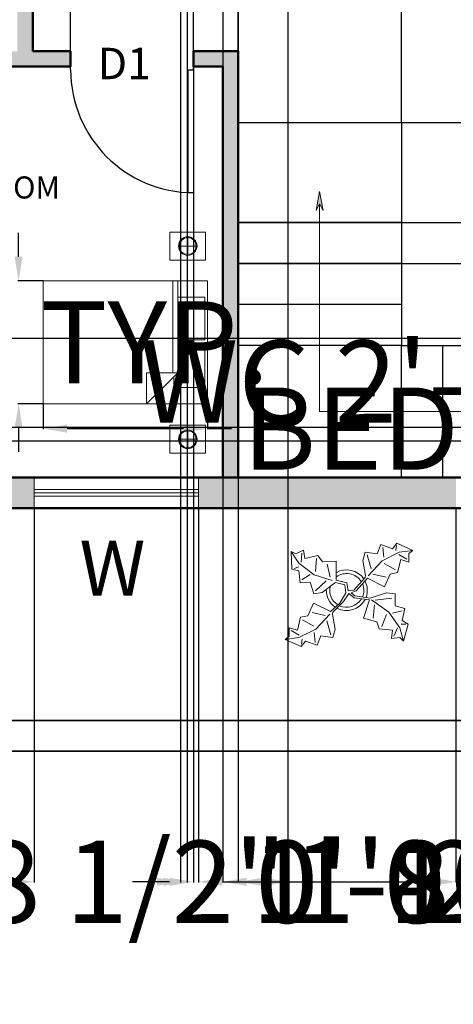
# Model space of a CAD drawing. Units: inches. Extents: x -166 to 1001, y 0 to 688.
# Tile 2 of 11: x 97 to 224, y 0 to 287. Entities that reach past the tile are written whole.
import ezdxf

# ---------------------------------------------------------------- set-up
doc = ezdxf.new("R2010")
doc.units = ezdxf.units.IN
doc.header["$MEASUREMENT"] = 0
for name, color, linetype, lineweight in [('A-ANNO-DIMS', 1, 'Continuous', 18), ('A-ANNO-SYMB', 7, 'Continuous', 18), ('A-ANNO-TEXT', 2, 'Continuous', 25), ('A-AREA-IDEN', 2, 'Continuous', 25), ('A-DOOR', 6, 'Continuous', 25), ('A-FLOR-STRS', 7, 'Continuous', 25), ('A-GLAZ', 130, 'Continuous', 18), ('A-WALL-PATT', 5, 'Continuous', 13), ('C-SITE-WALL', 250, 'Continuous', 35), ('FURNITURE', 11, 'Continuous', 18), ('TREES', 80, 'Continuous', 13), ('WALLS', 250, 'Continuous', 50)]:
    doc.layers.add(name, color=color, linetype=linetype, lineweight=lineweight)
doc.styles.get("Standard").update_dxf_attribs({"font": 'arial.ttf'})
doc.dimstyles.get("Standard").update_dxf_attribs({"dimtxt": 24, "dimasz": 7, "dimexe": 0.18, "dimexo": 0.0625, "dimgap": 0.09, "dimtad": 0, "dimtih": 1, "dimtoh": 1, "dimdec": 0, "dimzin": 0, "dimdsep": 46, "dimlunit": 3, "dimtxsty": 'Standard', "dimcen": 0.09, "dimadec": 0, "dimazin": 0, "dimtfac": 1, "dimtdec": 0, "dimtofl": 0, "dimtmove": 0, "dimatfit": 3, "dimfxl": 1, "dimtolj": 1, "dimtzin": 0, "dimarcsym": 0})

# ---------------------------------------------------------------- blocks, each defined once
blk = doc.blocks.new('*U6')
for p, q in [((0, 0), (0, -6)), ((40, 0), (40, -6))]:
    blk.add_line(p, q)
blk.add_lwpolyline([(0, 0), (0, 40), (1.75, 40), (1.75, 0)], close=True)
blk.add_arc((0, 0), 40, 0, 90)
blk = doc.blocks.new('Bed - Queen')
for p, q in [((0, -80.00003), (0, 0)), ((0, 0), (59.99999, 0)), ((59.99999, 0), (59.99999, -80.00003)), ((7.99999, -1.2), (28.79998, -1.2)), ((7.99999, -14.4), (7.99999, -1.2)), ((28.79998, -1.2), (28.79998, -14.4)), ((31.19999, -1.2), (51.99999, -1.2)), ((31.19999, -14.4), (31.19999, -1.2)), ((51.99999, -1.2), (51.99999, -16.4)), ((0, -14.4), (44.8, -14.4)), ((44.8, -16.8), (0, -16.8)), ((59.99999, -29.6), (44.8, -14.4)), ((44.8, -14.4), (44.8, -29.6)), ((51.99999, -16.4), (46.79936, -16.4)), ((44.8, -29.6), (59.99999, -29.6)), ((59.99999, -80.00003), (0, -80.00003))]:
    blk.add_line(p, q)
blk = doc.blocks.new('Plant - Rubber or Philodendron')
for p, q in [((-14.8639, 10.7964), (-12.6195, 11.8975)), ((-12.6195, 11.8975), (-12.1909, 9.4345)), ((8.8871, 10.7908), (9.9809, 13.4933)), ((9.9809, 13.4933), (13.3837, 12.301)), ((10.5828, 12.6946), (10.8893, 9.7953)), ((13.3837, 12.301), (14.68, 13.9039)), ((14.5816, 13.2037), (14.3848, 11.8033)), ((14.68, 13.9039), (19.3848, 11.8146)), ((19.3848, 11.8146), (15.3859, 11.3055)), ((19.3848, 11.8146), (18.1868, 10.9119)), ((-16.2005, 11.4774), (-13.9899, 8.1064)), ((-16.2005, 11.4774), (-14.8639, 10.7964)), ((-16.0159, 6.3329), (-16.2005, 11.4774)), ((-13.3174, 8.325), (-13.0735, 11.0065)), ((-12.1909, 9.4345), (-8.3829, 10.3)), ((-8.8369, 9.409), (-9.0894, 5.6095)), ((-8.3829, 10.3), (-7.0549, 8.501)), ((-7.0549, 8.501), (-3.0284, 8.6941)), ((-3.0284, 8.6941), (-3.0709, 3.1041)), ((4.6914, 8.8812), (5.3859, 11.2828)), ((4.6914, 8.8812), (5.5014, 4.4831)), ((5.3859, 11.2828), (8.8871, 10.7908)), ((5.9878, 10.4842), (7.1971, 6.3869)), ((10.3916, 8.7942), (6.2847, 4.4028)), ((15.3859, 11.3055), (10.3916, 8.7942)), ((15.7909, 9.1065), (14.8995, 5.3044)), ((15.2875, 10.6053), (17.5907, 9.2105)), ((18.1925, 8.4119), (15.7909, 9.1065)), ((18.1868, 10.9119), (18.1925, 8.4119)), ((-14.0069, 5.8704), (-16.0159, 6.3329)), ((-15.3434, 6.5514), (-13.9984, 6.9884)), ((-13.5868, 2.2894), (-14.0069, 5.8704)), ((-13.9899, 8.1064), (-9.5434, 4.7185)), ((-4.8529, 4.012), (-5.7184, 7.82)), ((14.2977, 6.1031), (10.9934, 7.9956)), ((-13.1329, 3.1804), (-10.6614, 4.727)), ((-9.5434, 4.7185), (-4.1917, 2.9888)), ((-9.1318, 0.0195), (-5.9793, 2.9025)), ((-3.0709, 3.1041), (0.0797, 2.3163)), ((2.1141, 0.2298), (5.4346, 3.9146)), ((6.1032, 3.6844), (2.8262, -0.031)), ((5.4346, 3.9146), (5.5014, 4.4831)), ((11.1089, 1.1958), (6.1032, 3.6844)), ((7.7005, 4.8881), (11.5025, 3.9967)), ((12.7005, 4.8994), (11.1089, 1.1958)), ((14.8995, 5.3044), (12.7005, 4.8994)), ((-10.6784, 2.491), (-13.5868, 2.2894)), ((-9.5858, -0.8715), (-10.6784, 2.491)), ((-7.1228, -0.443), (-3.5248, 2.2131)), ((-3.5248, 2.2131), (-3.3011, 2.4355)), ((-3.3011, 2.4355), (-0.5306, 1.7947)), ((-0.5306, 1.7947), (-0.2255, -0.5527)), ((-0.5306, 1.7947), (-0.5306, 1.7947)), ((0.0797, 2.3163), (0.4866, -0.031)), ((0.4866, -0.031), (2.1141, 0.2298)), ((-7.1228, -0.443), (-9.5858, -0.8715)), ((-2.019, -3.6148), (-0.2255, -0.5527)), ((-0.9375, -3.1608), (0.5883, -0.8135)), ((0.5883, -0.8135), (2.2447, -2.0916)), ((2.8262, -0.031), (1.3003, -0.5527)), ((1.3003, -0.5527), (2.4193, -1.4655)), ((2.2447, -2.0916), (6.7108, -2.6626)), ((2.4193, -1.4655), (6.895, -2.1175)), ((4.943, -7.9659), (6.7108, -2.6626)), ((11.6605, -0.5413), (6.895, -2.1175)), ((12.3677, -6.1981), (7.219, -2.6772)), ((8.3544, -2.7453), (13.1973, -2.1704)), ((11.6605, -0.5413), (14.1354, -0.8948)), ((14.1354, -0.8948), (14.1354, -4.4304)), ((-11.3237, -7.2629), (-9.7321, -3.5593)), ((-9.7321, -3.5593), (-4.7264, -6.0479)), ((-2.019, -3.6148), (-4.7264, -6.0479)), ((-4.0579, -6.2781), (-0.9375, -3.1608)), ((8.125, -4.0768), (7.7715, -7.9659)), ((14.1354, -4.4304), (16.9638, -5.1375)), ((16.9638, -5.1375), (16.2567, -8.673)), ((-14.4141, -11.4699), (-13.5228, -7.6679)), ((-13.5228, -7.6679), (-11.3237, -7.2629)), ((-12.921, -8.4665), (-9.6166, -10.359)), ((-6.3237, -7.2516), (-10.1257, -6.3602)), ((-9.0148, -11.1577), (-4.9047, -6.8122)), ((-4.1246, -6.8466), (-4.0579, -6.2781)), ((-3.3146, -11.2447), (-4.1246, -6.8466)), ((8.8321, -9.0266), (4.943, -7.9659)), ((10.2463, -10.4408), (11.6605, -6.9053)), ((15.5496, -10.7943), (12.3677, -6.1981)), ((16.2567, -5.8446), (13.4283, -6.5517)), ((-16.8157, -10.7754), (-14.4141, -11.4699)), ((-16.8101, -13.2754), (-16.8157, -10.7754)), ((-14.0091, -13.669), (-9.0148, -11.1577)), ((-4.611, -12.8477), (-5.8203, -8.7504)), ((-3.3146, -11.2447), (-4.0092, -13.6463)), ((9.5392, -11.1479), (8.8321, -9.0266)), ((13.4283, -11.5015), (9.5392, -11.1479)), ((13.0748, -13.9763), (13.4283, -11.5015)), ((14.8425, -10.7943), (13.7819, -13.2692)), ((16.6103, -14.6834), (15.5496, -10.7943)), ((17.3174, -9.7337), (15.9032, -9.7337)), ((16.2567, -8.673), (18.0245, -9.7337)), ((18.0245, -9.7337), (16.6103, -14.6834)), ((-18.008, -14.1781), (-16.8101, -13.2754)), ((-18.008, -14.1781), (-14.0091, -13.669)), ((-13.3032, -16.2674), (-18.008, -14.1781)), ((-13.9107, -12.9688), (-16.2139, -11.574)), ((-13.2048, -15.5672), (-13.008, -14.1668)), ((-9.206, -15.0581), (-9.5126, -12.1588)), ((-7.5103, -13.1543), (-8.6042, -15.8568)), ((-4.0092, -13.6463), (-7.5103, -13.1543)), ((15.5496, -13.6228), (13.0748, -13.9763)), ((16.6103, -14.6834), (15.5496, -13.6228)), ((-12.0069, -14.6645), (-13.3032, -16.2674)), ((-8.6042, -15.8568), (-12.0069, -14.6645))]:
    blk.add_line(p, q)
for centre, radius, start, end in [((0, 0), 6.1275, 34.37569, 120.1028), ((-0.0601, -0.2075), 5.2461, 33.82192, 124.9414), ((0.0308, 0.1664), 6, 178.6147, 235.1169), ((0.0308, 0.1664), 5, 168.1647, 238.6725), ((-0.2664, 0.1682), 5.2775, 338.4094, 20.03007), ((-0.098, 0.1364), 6.1288, 341.2017, 26.09184), ((-0.0234, 0.3825), 6.1492, 242.5812, 331.2714), ((-0.1102, 0.4886), 5.2883, 247.3711, 327.472)]:
    blk.add_arc(centre, radius, start, end)
blk = doc.blocks.new('WIN-48IN')
for p, q in [((0, 4.5), (0, 9)), ((0, 9), (0, 0)), ((48, 9), (48, 0)), ((0, 5.5), (48, 5.5)), ((0, 4.5), (48, 4.5)), ((0, 3.5), (48, 3.5))]:
    blk.add_line(p, q)
blk = doc.blocks.new('BEDSIDE-TABLE-LAMP')
for p, q in [((5.2, 1.64), (5.2, 6.55)), ((2.75, 4.1), (7.66, 4.1))]:
    blk.add_line(p, q)
blk.add_lwpolyline([(0, 8.19), (10.4, 8.19), (10.4, 0), (0, 0)], close=True)
for radius in [2.71, 2.71, 2.71, 2.46]:
    blk.add_circle((5.2, 4.1), radius)
blk = doc.blocks.new('*D23')
at = {"layer": 'A-ANNO-DIMS', "color": 0, "lineweight": -2, "transparency": 16777216}
for p, q in [((103.92, 175.12), (103.92, 167.8)), ((151.92, 175.12), (151.92, 167.8)), ((110.92, 167.98), (144.92, 167.98)), ((151.92, 167.98), (158.92, 167.98))]:
    blk.add_line(p, q, dxfattribs=at)
at = {"layer": 'A-ANNO-DIMS', "color": 0, "transparency": 16777216}
for points in [[(110.92, 169.15), (110.92, 166.82), (103.92, 167.98)], [(144.92, 169.15), (144.92, 166.82), (151.92, 167.98)]]:
    blk.add_solid(points, dxfattribs=at)
at = {"layer": 'Defpoints', "color": 0, "transparency": 16777216}
for p in [(103.92, 175.18), (151.92, 175.18), (151.92, 167.98)]:
    blk.add_point(p, dxfattribs=at)
at = {"layer": 'A-ANNO-DIMS', "color": 0, "transparency": 16777216, "insert": (270.75, 167.98), "char_height": 24, "attachment_point": 5}
blk.add_mtext('\\A1;BED 4\'-0" TYP.', dxfattribs=at)
blk = doc.blocks.new('*D24')
at = {"layer": 'A-ANNO-DIMS', "color": 0, "lineweight": -2, "transparency": 16777216}
for p, q in [((96.72, 218.18), (96.72, 225.18)), ((103.86, 211.18), (96.54, 211.18)), ((103.86, 175.18), (96.54, 175.18)), ((96.72, 168.18), (96.72, 161.18))]:
    blk.add_line(p, q, dxfattribs=at)
at = {"layer": 'A-ANNO-DIMS', "color": 0, "transparency": 16777216}
for points in [[(95.56, 218.18), (97.89, 218.18), (96.72, 211.18)], [(95.56, 168.18), (97.89, 168.18), (96.72, 175.18)]]:
    blk.add_solid(points, dxfattribs=at)
at = {"layer": 'Defpoints', "color": 0, "transparency": 16777216}
for p in [(103.92, 211.18), (96.72, 175.18), (103.92, 175.18)]:
    blk.add_point(p, dxfattribs=at)
at = {"layer": 'A-ANNO-DIMS', "color": 0, "transparency": 16777216, "insert": (96.72, 193.18), "char_height": 24, "attachment_point": 5}
blk.add_mtext('\\A1;3\'-0" TYP.', dxfattribs=at)
blk = doc.blocks.new('*D27')
at = {"layer": 'A-ANNO-DIMS', "color": 0, "lineweight": -2, "transparency": 16777216}
for p, q in [((325.13, 181.76), (318.13, 181.76)), ((325.13, 177.86), (325.13, 181.94)), ((344.51, 181.76), (332.13, 181.76)), ((351.51, 177.86), (351.51, 181.94))]:
    blk.add_line(p, q, dxfattribs=at)
at = {"layer": 'A-ANNO-DIMS', "color": 0, "transparency": 16777216}
for points in [[(332.13, 182.92), (332.13, 180.59), (325.13, 181.76)], [(344.51, 182.92), (344.51, 180.59), (351.51, 181.76)]]:
    blk.add_solid(points, dxfattribs=at)
at = {"layer": 'Defpoints', "color": 0, "transparency": 16777216}
for p in [(325.13, 181.76), (325.13, 177.8), (351.51, 177.8)]:
    blk.add_point(p, dxfattribs=at)
at = {"layer": 'A-ANNO-DIMS', "color": 0, "transparency": 16777216, "insert": (225.11, 181.76), "char_height": 24, "attachment_point": 5}
blk.add_mtext('\\A1;WC 2\'-2 1/2"', dxfattribs=at)
blk = doc.blocks.new('*D43')
at = {"layer": 'A-ANNO-DIMS', "color": 0, "lineweight": -2, "transparency": 16777216}
for p, q in [((160.88, 257.49), (160.88, 593.07)), ((167.88, 592.89), (201.62, 592.89)), ((208.62, 257.49), (208.62, 593.07)), ((208.62, 592.89), (215.62, 592.89))]:
    blk.add_line(p, q, dxfattribs=at)
at = {"layer": 'A-ANNO-DIMS', "color": 0, "transparency": 16777216}
for points in [[(167.88, 594.06), (167.88, 591.72), (160.88, 592.89)], [(201.62, 594.06), (201.62, 591.72), (208.62, 592.89)]]:
    blk.add_solid(points, dxfattribs=at)
at = {"layer": 'Defpoints', "color": 0, "transparency": 16777216}
for p in [(208.62, 592.89), (160.88, 257.42), (208.62, 257.42)]:
    blk.add_point(p, dxfattribs=at)
at = {"layer": 'A-ANNO-DIMS', "color": 0, "transparency": 16777216, "insert": (284.89, 592.89), "char_height": 24, "attachment_point": 5}
blk.add_mtext('\\A1;3\'-11 1/2"', dxfattribs=at)
blk = doc.blocks.new('*D44')
at = {"layer": 'A-ANNO-DIMS', "color": 0, "lineweight": -2, "transparency": 16777216}
for p, q in [((144.05, 474.68), (144.05, 35.41)), ((156.38, 474.68), (156.38, 35.41)), ((137.05, 35.59), (130.05, 35.59)), ((163.38, 35.59), (170.38, 35.59))]:
    blk.add_line(p, q, dxfattribs=at)
at = {"layer": 'A-ANNO-DIMS', "color": 0, "transparency": 16777216}
for points in [[(137.05, 36.76), (137.05, 34.42), (144.05, 35.59)], [(163.38, 36.76), (163.38, 34.42), (156.38, 35.59)]]:
    blk.add_solid(points, dxfattribs=at)
at = {"layer": 'Defpoints', "color": 0, "transparency": 16777216}
for p in [(144.05, 474.74), (156.38, 474.74), (156.38, 35.59)]:
    blk.add_point(p, dxfattribs=at)
at = {"layer": 'A-ANNO-DIMS', "color": 0, "transparency": 16777216, "insert": (229.2, 35.59), "char_height": 24, "attachment_point": 5}
blk.add_mtext('\\A1;1\'-0 1/2"', dxfattribs=at)
blk = doc.blocks.new('*D45')
at = {"layer": 'A-ANNO-DIMS', "color": 0, "lineweight": -2, "transparency": 16777216}
for p, q in [((160.88, 474.68), (160.88, 35.41)), ((175.47, 474.68), (175.47, 35.41)), ((167.88, 35.59), (168.47, 35.59)), ((175.47, 35.59), (182.47, 35.59))]:
    blk.add_line(p, q, dxfattribs=at)
at = {"layer": 'A-ANNO-DIMS', "color": 0, "transparency": 16777216}
for points in [[(167.88, 36.76), (167.88, 34.42), (160.88, 35.59)], [(168.47, 36.76), (168.47, 34.42), (175.47, 35.59)]]:
    blk.add_solid(points, dxfattribs=at)
at = {"layer": 'Defpoints', "color": 0, "transparency": 16777216}
for p in [(160.88, 474.74), (175.47, 474.74), (175.47, 35.59)]:
    blk.add_point(p, dxfattribs=at)
at = {"layer": 'A-ANNO-DIMS', "color": 0, "transparency": 16777216, "insert": (241.29, 35.59), "char_height": 24, "attachment_point": 5}
blk.add_mtext('\\A1;1\'-2 1/2"', dxfattribs=at)
blk = doc.blocks.new('*D48')
at = {"layer": 'A-ANNO-DIMS', "color": 0, "lineweight": -2, "transparency": 16777216}
for p, q in [((15.38, 144.68), (15.38, 35.41)), ((101.31, 144.68), (101.31, 35.41)), ((22.38, 35.59), (26.46, 35.59)), ((94.31, 35.59), (90.24, 35.59))]:
    blk.add_line(p, q, dxfattribs=at)
at = {"layer": 'A-ANNO-DIMS', "color": 0, "transparency": 16777216}
for points in [[(22.38, 36.76), (22.38, 34.42), (15.38, 35.59)], [(94.31, 36.76), (94.31, 34.42), (101.31, 35.59)]]:
    blk.add_solid(points, dxfattribs=at)
at = {"layer": 'Defpoints', "color": 0, "transparency": 16777216}
for p in [(15.38, 144.74), (101.31, 144.74), (101.31, 35.59)]:
    blk.add_point(p, dxfattribs=at)
at = {"layer": 'A-ANNO-DIMS', "color": 0, "transparency": 16777216, "insert": (58.35, 35.59), "char_height": 24, "attachment_point": 5}
blk.add_mtext('\\A1;7\'-2"', dxfattribs=at)
blk = doc.blocks.new('*D49')
at = {"layer": 'A-ANNO-DIMS', "color": 0, "lineweight": -2, "transparency": 16777216}
for p, q in [((149.31, 144.68), (149.31, 35.41)), ((224.58, 144.68), (224.58, 35.41)), ((156.31, 35.59), (217.58, 35.59)), ((224.58, 35.59), (231.58, 35.59))]:
    blk.add_line(p, q, dxfattribs=at)
at = {"layer": 'A-ANNO-DIMS', "color": 0, "transparency": 16777216}
for points in [[(156.31, 36.76), (156.31, 34.42), (149.31, 35.59)], [(217.58, 36.76), (217.58, 34.42), (224.58, 35.59)]]:
    blk.add_solid(points, dxfattribs=at)
at = {"layer": 'Defpoints', "color": 0, "transparency": 16777216}
for p in [(149.31, 144.74), (224.58, 144.74), (224.58, 35.59)]:
    blk.add_point(p, dxfattribs=at)
at = {"layer": 'A-ANNO-DIMS', "color": 0, "transparency": 16777216, "insert": (291.6, 35.59), "char_height": 24, "attachment_point": 5}
blk.add_mtext('\\A1;6\'-3 1/2"', dxfattribs=at)
blk = doc.blocks.new('*D51')
at = {"layer": 'A-ANNO-DIMS', "color": 0, "lineweight": -2, "transparency": 16777216}
for p, q in [((675.03, 168.41), (675.03, 175.41)), ((675.03, 175.41), (682.03, 175.41)), ((24.44, 168.41), (675.21, 168.41)), ((675.03, 160.74), (675.03, 161.41)), ((24.44, 153.74), (675.21, 153.74))]:
    blk.add_line(p, q, dxfattribs=at)
at = {"layer": 'A-ANNO-DIMS', "color": 0, "transparency": 16777216}
for points in [[(673.87, 161.41), (676.2, 161.41), (675.03, 168.41)], [(673.87, 160.74), (676.2, 160.74), (675.03, 153.74)]]:
    blk.add_solid(points, dxfattribs=at)
at = {"layer": 'Defpoints', "color": 0, "transparency": 16777216}
for p in [(24.38, 168.41), (675.03, 168.41), (24.38, 153.74)]:
    blk.add_point(p, dxfattribs=at)
at = {"layer": 'A-ANNO-DIMS', "color": 0, "transparency": 16777216, "insert": (740.85, 175.41), "char_height": 24, "attachment_point": 5}
blk.add_mtext('\\A1;1\'-2 1/2"', dxfattribs=at)
blk = doc.blocks.new('*D55')
at = {"layer": 'A-ANNO-DIMS', "color": 0, "lineweight": -2, "transparency": 16777216}
for p, q in [((-120.77, 341.73), (-120.77, 348.73)), ((529.82, 334.73), (-120.95, 334.73)), ((529.82, 298.79), (-120.95, 298.79)), ((-120.77, 291.79), (-120.77, 284.79))]:
    blk.add_line(p, q, dxfattribs=at)
at = {"layer": 'A-ANNO-DIMS', "color": 0, "transparency": 16777216}
for points in [[(-121.93, 341.73), (-119.6, 341.73), (-120.77, 334.73)], [(-121.93, 291.79), (-119.6, 291.79), (-120.77, 298.79)]]:
    blk.add_solid(points, dxfattribs=at)
at = {"layer": 'Defpoints', "color": 0, "transparency": 16777216}
for p in [(-120.77, 334.73), (529.88, 334.73), (529.88, 298.79)]:
    blk.add_point(p, dxfattribs=at)
at = {"layer": 'A-ANNO-DIMS', "color": 0, "transparency": 16777216, "insert": (-120.77, 316.76), "char_height": 24, "attachment_point": 5}
blk.add_mtext('\\A1;3\'-0"', dxfattribs=at)
blk = doc.blocks.new('*D60')
at = {"layer": 'A-ANNO-DIMS', "color": 0, "lineweight": -2, "transparency": 16777216}
for p, q in [((156.38, 342.68), (156.38, 35.41)), ((146.03, 338.18), (146.03, 35.41)), ((139.03, 35.59), (132.03, 35.59)), ((163.38, 35.59), (170.38, 35.59))]:
    blk.add_line(p, q, dxfattribs=at)
at = {"layer": 'A-ANNO-DIMS', "color": 0, "transparency": 16777216}
for points in [[(139.03, 36.76), (139.03, 34.42), (146.03, 35.59)], [(163.38, 36.76), (163.38, 34.42), (156.38, 35.59)]]:
    blk.add_solid(points, dxfattribs=at)
at = {"layer": 'Defpoints', "color": 0, "transparency": 16777216}
for p in [(156.38, 342.74), (146.03, 338.24), (156.38, 35.59)]:
    blk.add_point(p, dxfattribs=at)
at = {"layer": 'A-ANNO-DIMS', "color": 0, "transparency": 16777216, "insert": (239.66, 35.59), "char_height": 24, "attachment_point": 5}
blk.add_mtext('\\A1;0\'-10 1/2"', dxfattribs=at)
blk = doc.blocks.new('*D67')
at = {"layer": 'A-ANNO-DIMS', "color": 0, "lineweight": -2, "transparency": 16777216}
for p, q in [((44.93, 278.3), (44.93, 593.07)), ((51.93, 592.89), (67.93, 592.89)), ((74.93, 278.3), (74.93, 593.07)), ((74.93, 592.89), (81.93, 592.89))]:
    blk.add_line(p, q, dxfattribs=at)
at = {"layer": 'A-ANNO-DIMS', "color": 0, "transparency": 16777216}
for points in [[(51.93, 594.06), (51.93, 591.72), (44.93, 592.89)], [(67.93, 594.06), (67.93, 591.72), (74.93, 592.89)]]:
    blk.add_solid(points, dxfattribs=at)
at = {"layer": 'Defpoints', "color": 0, "transparency": 16777216}
for p in [(74.93, 592.89), (44.93, 278.24), (74.93, 278.24)]:
    blk.add_point(p, dxfattribs=at)
at = {"layer": 'A-ANNO-DIMS', "color": 0, "transparency": 16777216, "insert": (114.12, 592.89), "char_height": 24, "attachment_point": 5}
blk.add_mtext('\\A1;2\'-6"', dxfattribs=at)
blk = doc.blocks.new('*D68')
at = {"layer": 'A-ANNO-DIMS', "color": 0, "lineweight": -2, "transparency": 16777216}
for p, q in [((24.38, 273.68), (24.38, 35.41)), ((44.93, 273.68), (44.93, 35.41)), ((31.38, 35.59), (37.93, 35.59)), ((44.93, 35.59), (51.93, 35.59))]:
    blk.add_line(p, q, dxfattribs=at)
at = {"layer": 'A-ANNO-DIMS', "color": 0, "transparency": 16777216}
for points in [[(31.38, 36.76), (31.38, 34.42), (24.38, 35.59)], [(37.93, 36.76), (37.93, 34.42), (44.93, 35.59)]]:
    blk.add_solid(points, dxfattribs=at)
at = {"layer": 'Defpoints', "color": 0, "transparency": 16777216}
for p in [(24.38, 273.74), (44.93, 273.74), (44.93, 35.59)]:
    blk.add_point(p, dxfattribs=at)
at = {"layer": 'A-ANNO-DIMS', "color": 0, "transparency": 16777216, "insert": (110.75, 35.59), "char_height": 24, "attachment_point": 5}
blk.add_mtext('\\A1;1\'-8 1/2"', dxfattribs=at)
blk = doc.blocks.new('*D69')
at = {"layer": 'A-ANNO-DIMS', "color": 0, "lineweight": -2, "transparency": 16777216}
for p, q in [((111.92, 278.3), (111.92, 593.07)), ((118.92, 592.89), (140.87, 592.89)), ((147.87, 278.3), (147.87, 593.07)), ((147.87, 592.89), (154.87, 592.89))]:
    blk.add_line(p, q, dxfattribs=at)
at = {"layer": 'A-ANNO-DIMS', "color": 0, "transparency": 16777216}
for points in [[(118.92, 594.06), (118.92, 591.72), (111.92, 592.89)], [(140.87, 594.06), (140.87, 591.72), (147.87, 592.89)]]:
    blk.add_solid(points, dxfattribs=at)
at = {"layer": 'Defpoints', "color": 0, "transparency": 16777216}
for p in [(147.87, 592.89), (111.92, 278.24), (147.87, 278.24)]:
    blk.add_point(p, dxfattribs=at)
at = {"layer": 'A-ANNO-DIMS', "color": 0, "transparency": 16777216, "insert": (186.85, 592.89), "char_height": 24, "attachment_point": 5}
blk.add_mtext('\\A1;3\'-0"', dxfattribs=at)
blk = doc.blocks.new('*D70')
at = {"layer": 'A-ANNO-DIMS', "color": 0, "lineweight": -2, "transparency": 16777216}
for p, q in [((147.87, 273.68), (147.87, 35.41)), ((156.38, 273.68), (156.38, 35.41)), ((140.87, 35.59), (133.87, 35.59)), ((163.38, 35.59), (170.38, 35.59))]:
    blk.add_line(p, q, dxfattribs=at)
at = {"layer": 'A-ANNO-DIMS', "color": 0, "transparency": 16777216}
for points in [[(140.87, 36.76), (140.87, 34.42), (147.87, 35.59)], [(163.38, 36.76), (163.38, 34.42), (156.38, 35.59)]]:
    blk.add_solid(points, dxfattribs=at)
at = {"layer": 'Defpoints', "color": 0, "transparency": 16777216}
for p in [(147.87, 273.74), (156.38, 273.74), (156.38, 35.59)]:
    blk.add_point(p, dxfattribs=at)
at = {"layer": 'A-ANNO-DIMS', "color": 0, "transparency": 16777216, "insert": (230.33, 35.59), "char_height": 24, "attachment_point": 5}
blk.add_mtext('\\A1;0\'-8 1/2"', dxfattribs=at)
blk = doc.blocks.new('*D73')
at = {"layer": 'A-ANNO-DIMS', "color": 0, "lineweight": -2, "transparency": 16777216}
for p, q in [((-120.77, 201.32), (-120.77, 208.32)), ((393.32, 194.32), (-120.95, 194.32)), ((393.32, 164.32), (-120.95, 164.32)), ((-120.77, 157.32), (-120.77, 150.32))]:
    blk.add_line(p, q, dxfattribs=at)
at = {"layer": 'A-ANNO-DIMS', "color": 0, "transparency": 16777216}
for points in [[(-121.93, 201.32), (-119.6, 201.32), (-120.77, 194.32)], [(-121.93, 157.32), (-119.6, 157.32), (-120.77, 164.32)]]:
    blk.add_solid(points, dxfattribs=at)
at = {"layer": 'Defpoints', "color": 0, "transparency": 16777216}
for p in [(-120.77, 194.32), (393.38, 194.32), (393.38, 164.32)]:
    blk.add_point(p, dxfattribs=at)
at = {"layer": 'A-ANNO-DIMS', "color": 0, "transparency": 16777216, "insert": (-120.77, 179.32), "char_height": 24, "attachment_point": 5}
blk.add_mtext('\\A1;2\'-6"', dxfattribs=at)
blk = doc.blocks.new('*D76')
at = {"layer": 'A-ANNO-DIMS', "color": 0, "lineweight": -2, "transparency": 16777216}
for p, q in [((675.03, 235.24), (675.03, 242.24)), ((160.94, 228.24), (675.21, 228.24)), ((160.94, 216.24), (675.21, 216.24)), ((675.03, 209.24), (675.03, 202.24)), ((675.03, 202.24), (668.03, 202.24))]:
    blk.add_line(p, q, dxfattribs=at)
at = {"layer": 'A-ANNO-DIMS', "color": 0, "transparency": 16777216}
for points in [[(673.87, 235.24), (676.2, 235.24), (675.03, 228.24)], [(673.87, 209.24), (676.2, 209.24), (675.03, 216.24)]]:
    blk.add_solid(points, dxfattribs=at)
at = {"layer": 'Defpoints', "color": 0, "transparency": 16777216}
for p in [(160.88, 228.24), (160.88, 216.24), (675.03, 216.24)]:
    blk.add_point(p, dxfattribs=at)
at = {"layer": 'A-ANNO-DIMS', "color": 0, "transparency": 16777216, "insert": (637.17, 202.24), "char_height": 24, "attachment_point": 5}
blk.add_mtext('\\A1;1\'-0"', dxfattribs=at)
blk = doc.blocks.new('*D78')
at = {"layer": 'A-ANNO-DIMS', "color": 0, "lineweight": -2, "transparency": 16777216}
for p, q in [((160.88, 153.8), (160.88, 593.07)), ((167.88, 592.89), (186.64, 592.89)), ((285.77, 592.89), (267.01, 592.89)), ((292.77, 153.8), (292.77, 593.07))]:
    blk.add_line(p, q, dxfattribs=at)
at = {"layer": 'A-ANNO-DIMS', "color": 0, "transparency": 16777216}
for points in [[(167.88, 594.06), (167.88, 591.72), (160.88, 592.89)], [(285.77, 594.06), (285.77, 591.72), (292.77, 592.89)]]:
    blk.add_solid(points, dxfattribs=at)
at = {"layer": 'Defpoints', "color": 0, "transparency": 16777216}
for p in [(292.77, 592.89), (160.88, 153.74), (292.77, 153.74)]:
    blk.add_point(p, dxfattribs=at)
at = {"layer": 'A-ANNO-DIMS', "color": 0, "transparency": 16777216, "insert": (226.83, 592.89), "char_height": 24, "attachment_point": 5}
blk.add_mtext('\\A1;11\'-0"', dxfattribs=at)
blk = doc.blocks.new('*D79')
at = {"layer": 'A-ANNO-DIMS', "color": 0, "lineweight": -2, "transparency": 16777216}
for p, q in [((208.68, 257.42), (675.21, 257.42)), ((675.03, 250.42), (675.03, 218.08)), ((675.03, 160.74), (675.03, 193.08)), ((292.83, 153.74), (675.21, 153.74))]:
    blk.add_line(p, q, dxfattribs=at)
at = {"layer": 'A-ANNO-DIMS', "color": 0, "transparency": 16777216}
for points in [[(673.87, 250.42), (676.2, 250.42), (675.03, 257.42)], [(673.87, 160.74), (676.2, 160.74), (675.03, 153.74)]]:
    blk.add_solid(points, dxfattribs=at)
at = {"layer": 'Defpoints', "color": 0, "transparency": 16777216}
for p in [(208.62, 257.42), (292.77, 153.74), (675.03, 153.74)]:
    blk.add_point(p, dxfattribs=at)
at = {"layer": 'A-ANNO-DIMS', "color": 0, "transparency": 16777216, "insert": (675.03, 205.58), "char_height": 24, "attachment_point": 5}
blk.add_mtext('\\A1;8\'-7 1/2"', dxfattribs=at)

msp = doc.modelspace()

# ---------------------------------------------------------------- hatches: boundary and pattern name
at = {"layer": 'A-ANNO-SYMB'}
h = msp.add_hatch(color=256, dxfattribs=at)
h.dxf.hatch_style = 1
h.paths.add_polyline_path([(184.73, 237.23), (183.69, 231.68), (184.73, 233.61), (185.76, 231.68)])
at = {"layer": 'A-WALL-PATT'}
h = msp.add_hatch(color=256, dxfattribs=at)
h.dxf.hatch_style = 1
h.paths.add_polyline_path([(96.05, 483.74), (15.38, 483.74), (15.38, 414.29), (24.38, 414.29), (24.38, 474.74), (96.05, 474.74)])
h.paths.add_polyline_path([(175.47, 483.74), (144.05, 483.74), (144.05, 474.74), (156.38, 474.74), (175.47, 474.74)])
h.paths.add_polyline_path([(298.66, 483.74), (199.47, 483.74), (199.47, 474.74), (256.88, 474.74), (298.66, 474.74)])
h.paths.add_polyline_path([(430.46, 483.74), (346.66, 483.74), (346.66, 474.74), (393.38, 474.74), (430.46, 474.74)])
h.paths.add_polyline_path([(261.38, 474.74), (256.88, 474.74), (256.88, 342.74), (201.55, 342.74), (201.55, 338.24), (274.49, 338.24), (274.49, 342.74), (261.38, 342.74)])
h.paths.add_polyline_path([(160.88, 474.74), (156.38, 474.74), (156.38, 342.74), (146.03, 342.74), (146.03, 338.24), (171.55, 338.24), (171.55, 342.74), (160.88, 342.74)])
h.paths.add_polyline_path([(397.88, 474.74), (393.38, 474.74), (393.38, 383.21), (397.88, 383.21)])
h.paths.add_polyline_path([(538.88, 362.18), (529.88, 362.18), (529.88, 342.74), (397.88, 342.74), (397.88, 348.69), (393.38, 348.69), (393.38, 342.74), (384.24, 342.74), (384.24, 338.24), (529.88, 338.24), (529.88, 334.73), (538.88, 334.73)])
h.paths.add_polyline_path([(538.88, 483.74), (478.46, 483.74), (478.46, 474.74), (529.88, 474.74), (529.88, 410.18), (538.88, 410.18)])
h.paths.add_polyline_path([(538.88, 298.79), (529.88, 298.79), (529.88, 278.24), (442.61, 278.24), (442.61, 273.74), (529.88, 273.74), (529.88, 221.94), (538.88, 221.94)])
h.paths.add_polyline_path([(538.88, 173.94), (529.88, 173.94), (529.88, 153.74), (393.38, 153.74), (382.23, 153.74), (382.23, 144.74), (538.88, 144.74)])
h.paths.add_polyline_path([(397.88, 164.32), (393.38, 164.32), (393.38, 153.74), (397.88, 153.74)], flags=17)
h.paths.add_polyline_path([(397.88, 273.74), (406.66, 273.74), (406.66, 278.24), (393.38, 278.24), (393.38, 273.74), (393.38, 230.24), (316.88, 230.24), (316.88, 153.74), (321.38, 153.74), (321.38, 225.74), (393.38, 225.74), (393.38, 194.32), (397.88, 194.32)])
h.paths.add_polyline_path([(358.23, 153.74), (316.88, 153.74), (284.58, 153.74), (284.58, 144.74), (358.23, 144.74)])
h.paths.add_polyline_path([(224.58, 153.74), (156.38, 153.74), (149.31, 153.74), (149.31, 144.74), (224.58, 144.74)])
h.paths.add_polyline_path([(101.31, 153.74), (24.38, 153.74), (24.38, 168.41), (15.38, 168.41), (15.38, 144.74), (101.31, 144.74)])
h.paths.add_polyline_path([(160.88, 273.74), (160.88, 278.24), (147.87, 278.24), (147.87, 273.74), (156.38, 273.74), (156.38, 153.74), (160.88, 153.74)])
h.paths.add_polyline_path([(111.92, 278.24), (100.88, 278.24), (100.88, 338.24), (110.03, 338.24), (110.03, 342.74), (24.38, 342.74), (24.38, 366.29), (15.38, 366.29), (15.38, 216.41), (24.38, 216.41), (24.38, 273.74), (44.93, 273.74), (44.93, 278.24), (24.38, 278.24), (24.38, 338.24), (96.38, 338.24), (96.38, 278.24), (74.93, 278.24), (74.93, 273.74), (111.92, 273.74)])

# ---------------------------------------------------------------- linework, layer by layer
at = {"layer": 'A-ANNO-SYMB'}
for p, q in [((183.69, 231.68), (184.73, 237.23)), ((185.76, 231.68), (184.73, 237.23)), ((184.73, 233.61), (183.69, 231.68)), ((184.73, 172.99), (184.73, 233.61)), ((184.73, 233.61), (185.76, 231.68)), ((256.68, 172.99), (184.73, 172.99))]:
    msp.add_line(p, q, dxfattribs=at)
at = {"layer": 'A-FLOR-STRS'}
for p, q in [((160.88, 257.42), (208.62, 257.42)), ((208.62, 257.42), (208.62, 192.24)), ((208.57, 228.24), (160.88, 228.24)), ((208.57, 216.24), (160.88, 216.24)), ((208.57, 204.24), (160.88, 204.24)), ((208.57, 192.24), (160.88, 192.24)), ((208.57, 192.24), (208.57, 153.74)), ((208.62, 192.24), (292.77, 192.24)), ((220.6, 192.24), (220.6, 153.74))]:
    msp.add_line(p, q, dxfattribs=at)
at = {"layer": 'C-SITE-WALL'}
for p, q in [((-73.62, 82.74), (627.88, 82.74)), ((-82.62, 73.74), (636.88, 73.74))]:
    msp.add_line(p, q, dxfattribs=at)
at = {"layer": 'WALLS'}
for p, q in [((100.88, 278.24), (100.88, 338.24)), ((100.88, 278.24), (111.92, 278.24)), ((111.92, 278.24), (111.92, 273.74)), ((147.87, 273.74), (147.87, 278.24)), ((147.87, 278.24), (160.88, 278.24)), ((160.88, 273.74), (160.88, 278.24)), ((74.93, 273.74), (111.92, 273.74)), ((147.87, 273.74), (156.38, 273.74)), ((156.38, 153.74), (156.38, 273.74)), ((160.88, 153.74), (160.88, 273.74)), ((24.38, 153.74), (156.38, 153.74)), ((156.38, 153.74), (316.88, 153.74)), ((15.38, 144.74), (538.88, 144.74))]:
    msp.add_line(p, q, dxfattribs=at)

# ---------------------------------------------------------------- block references
at = {"layer": 'A-DOOR', "xscale": 0.8986699555462259, "yscale": 0.8986699555462259, "zscale": 0.8986699555462259, "rotation": 180}
msp.add_blockref('*U6', (147.87, 272.85), dxfattribs=at)
at = {"layer": 'A-GLAZ'}
msp.add_blockref('WIN-48IN', (101.31, 144.74), dxfattribs=at)
at = {"layer": 'FURNITURE'}
for p in [(140.97, 217.22), (140.97, 160.78)]:
    msp.add_blockref('BEDSIDE-TABLE-LAMP', p, dxfattribs=at)
at = {"layer": 'FURNITURE', "xscale": 0.6000001000000168, "yscale": 0.6000001000000168, "zscale": 0.6000001000000168, "rotation": 270}
msp.add_blockref('Bed - Queen', (151.92, 211.18), dxfattribs=at)
at = {"layer": 'TREES'}
msp.add_blockref('Plant - Rubber or Philodendron', (192.62, 120.6), dxfattribs=at)

# ---------------------------------------------------------------- texts
at = {"layer": 'A-ANNO-TEXT'}
for s, height, p in [('D1', 9.17, (119.85, 270.07)), ('W ', 16.096, (114.52, 119.14))]:
    msp.add_text(s, height=height, dxfattribs=at).set_placement(p)
at = {"layer": 'A-AREA-IDEN'}
msp.add_text('GUEST BEDROOM', height=6.4554, dxfattribs=at).set_placement((35.86, 235.21))

# ---------------------------------------------------------------- dimensions: what is measured, and where the dimension line sits
at = {"layer": 'A-ANNO-DIMS'}
for base, p1, p2, picture, middle in [((208.62, 592.89), (160.88, 257.42), (208.62, 257.42), '*D43', (284.89, 592.89)), ((74.93, 592.89), (44.93, 278.24), (74.93, 278.24), '*D67', (114.12, 592.89)), ((147.8711, 592.8909), (111.9243, 278.2409), (147.8711, 278.2409), '*D69', (186.852, 592.8909)), ((292.77, 592.89), (160.88, 153.74), (292.77, 153.74), '*D78', (226.83, 592.89)), ((156.38, 35.59), (144.05, 474.74), (156.38, 474.74), '*D44', (229.2, 35.59)), ((175.47, 35.59), (160.88, 474.74), (175.47, 474.74), '*D45', (241.29, 35.59)), ((156.3825, 35.5909), (146.0262, 338.2409), (156.3825, 342.7409), '*D60', (239.6566, 35.5909)), ((44.9284, 35.5909), (24.3825, 273.7409), (44.9284, 273.7409), '*D68', (110.7496, 35.5909)), ((156.38, 35.59), (147.87, 273.74), (156.38, 273.74), '*D70', (230.33, 35.59)), ((101.31, 35.59), (15.38, 144.74), (101.31, 144.74), '*D48', (58.35, 35.59)), ((224.58, 35.59), (149.31, 144.74), (224.58, 144.74), '*D49', (291.6, 35.59))]:
    dim = msp.add_linear_dim(base=base, p1=p1, p2=p2, dimstyle='Standard', override={"dimdec": 1, "dimlfac": 1, "dimrnd": 0, "dimzin": 1, "dimdsep": 46, "dimlunit": 4, "dimfrac": 2}, dxfattribs=at)
    dim.commit()
    dim.dimension.update_dxf_attribs({"geometry": picture, "text_midpoint": middle})
for base, p1, p2, picture, middle in [((-120.77, 334.73), (529.88, 298.79), (529.88, 334.73), '*D55', (-120.77, 316.76)), ((675.03, 153.74), (208.62, 257.42), (292.77, 153.74), '*D79', (675.03, 205.58)), ((675.03, 216.24), (160.88, 228.24), (160.88, 216.24), '*D76', (637.17, 202.24)), ((675.03, 168.41), (24.38, 153.74), (24.38, 168.41), '*D51', (740.85, 175.41)), ((-120.77, 194.32), (393.38, 164.32), (393.38, 194.32), '*D73', (-120.77, 179.32))]:
    dim = msp.add_linear_dim(base=base, p1=p1, p2=p2, angle=90, dimstyle='Standard', override={"dimdec": 1, "dimlfac": 1, "dimrnd": 0, "dimzin": 1, "dimdsep": 46, "dimlunit": 4, "dimfrac": 2}, dxfattribs=at)
    dim.commit()
    dim.dimension.update_dxf_attribs({"geometry": picture, "text_midpoint": middle})
for base, p1, p2, angle, text, picture, middle in [((325.13, 181.76), (351.51, 177.8), (325.13, 177.8), 180, 'WC <>', '*D27', (225.11, 181.76)), ((96.72, 175.18), (103.92, 211.18), (103.92, 175.18), 270, '<> TYP.', '*D24', (96.72, 193.18))]:
    dim = msp.add_linear_dim(base=base, p1=p1, p2=p2, angle=angle, text=text, dimstyle='Standard', override={"dimdec": 1, "dimlfac": 1, "dimrnd": 0, "dimzin": 1, "dimdsep": 46, "dimlunit": 4, "dimfrac": 2}, dxfattribs=at)
    dim.commit()
    dim.dimension.update_dxf_attribs({"geometry": picture, "text_midpoint": middle})
dim = msp.add_linear_dim(base=(151.92, 167.98), p1=(103.92, 175.18), p2=(151.92, 175.18), text='BED <> TYP.', dimstyle='Standard', override={"dimdec": 1, "dimlfac": 1, "dimrnd": 0, "dimzin": 1, "dimdsep": 46, "dimlunit": 4, "dimfrac": 2}, dxfattribs=at)
dim.commit()
dim.dimension.update_dxf_attribs({"geometry": '*D23', "text_midpoint": (270.75, 167.98)})

doc.saveas('drawing.dxf')
